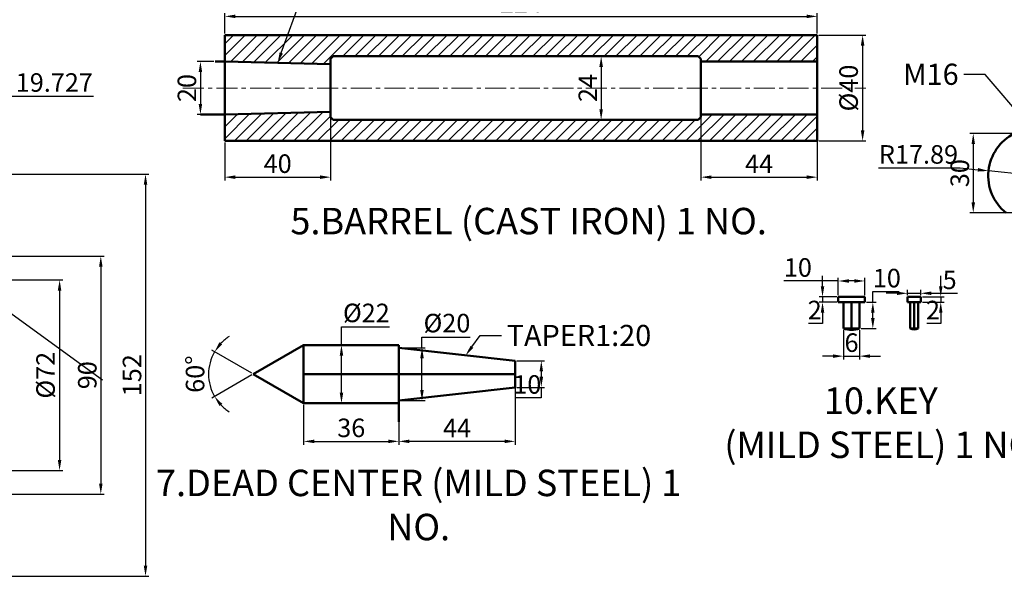
# Model space of a CAD drawing. Units: millimetres. Extents: x -66 to 1195, y -396 to 398.
# Tile 4 of 8: x 373 to 745, y -176 to 35. Entities that reach past the tile are written whole.
import ezdxf
from ezdxf import colors
from ezdxf.entities.mleader import LeaderData, LeaderLine
from ezdxf.math import Vec2, Vec3

# ---------------------------------------------------------------- set-up
doc = ezdxf.new("R2010")
doc.units = ezdxf.units.MM
doc.header["$LTSCALE"] = 0.5
doc.linetypes.add('CENTER', pattern=[50.8, 31.75, -6.35, 6.35, -6.35])
for name, color, linetype, lineweight in [('M-CNTR', 1, 'CENTER', 18), ('M-DIMS', 2, 'Continuous', 25), ('M-HATC', 8, 'Continuous', 18), ('M-OUTL', 7, 'Continuous', 50), ('M-TEXT', 7, 'Continuous', 25)]:
    doc.layers.add(name, color=color, linetype=linetype, lineweight=lineweight)
doc.styles.get("Standard").update_dxf_attribs({"font": 'arial.ttf'})
doc.dimstyles.new('ISO-25', dxfattribs={"dimtxt": 7, "dimasz": 4, "dimexe": 1.25, "dimexo": 0.625, "dimtad": 1, "dimtoh": 1, "dimtxsty": 'Standard', "dimcen": 2.5, "dimadec": 0, "dimazin": 0, "dimtfac": 1, "dimtmove": 0, "dimatfit": 3, "dimfxl": 1, "dimarcsym": 0})

# ---------------------------------------------------------------- blocks, each defined once
blk = doc.blocks.new('*D23')
at = {"layer": 'Defpoints', "color": 0, "ltscale": 0.5, "transparency": 16777216}
for p in [(346.94, -63.65), (346.94, -135.65), (387.75, -135.65)]:
    blk.add_point(p, dxfattribs=at)
at = {"layer": 'M-DIMS', "color": 0, "lineweight": -2, "ltscale": 0.5, "transparency": 16777216}
for p, q in [((347.56, -63.65), (389, -63.65)), ((387.75, -67.65), (387.75, -131.65)), ((347.56, -135.65), (389, -135.65))]:
    blk.add_line(p, q, dxfattribs=at)
at = {"layer": 'M-DIMS', "color": 0, "ltscale": 0.5, "transparency": 16777216}
for points in [[(387.08, -67.65), (388.41, -67.65), (387.75, -63.65)], [(387.08, -131.65), (388.41, -131.65), (387.75, -135.65)]]:
    blk.add_solid(points, dxfattribs=at)
at = {"layer": 'M-DIMS', "color": 0, "ltscale": 0.5, "transparency": 16777216, "insert": (383.35, -99.65), "char_height": 7, "attachment_point": 5, "rotation": 90}
blk.add_mtext('%%C72', dxfattribs=at)
blk = doc.blocks.new('*D24')
at = {"layer": 'Defpoints', "color": 0, "ltscale": 0.5, "transparency": 16777216}
for p in [(332.94, -54.65), (332.94, -144.65), (403.33, -144.65)]:
    blk.add_point(p, dxfattribs=at)
at = {"layer": 'M-DIMS', "color": 0, "lineweight": -2, "ltscale": 0.5, "transparency": 16777216}
for p, q in [((333.56, -54.65), (404.58, -54.65)), ((403.33, -58.65), (403.33, -140.65)), ((333.56, -144.65), (404.58, -144.65))]:
    blk.add_line(p, q, dxfattribs=at)
at = {"layer": 'M-DIMS', "color": 0, "ltscale": 0.5, "transparency": 16777216}
for points in [[(402.67, -58.65), (404, -58.65), (403.33, -54.65)], [(402.67, -140.65), (404, -140.65), (403.33, -144.65)]]:
    blk.add_solid(points, dxfattribs=at)
at = {"layer": 'M-DIMS', "color": 0, "ltscale": 0.5, "transparency": 16777216, "insert": (399.13, -99.65), "char_height": 7, "attachment_point": 5, "rotation": 90}
blk.add_mtext('90', dxfattribs=at)
blk = doc.blocks.new('*D25')
at = {"layer": 'Defpoints', "color": 0, "ltscale": 0.5, "transparency": 16777216}
for p in [(366.94, -23.65), (366.94, -175.65), (420.24, -175.65)]:
    blk.add_point(p, dxfattribs=at)
at = {"layer": 'M-DIMS', "color": 0, "lineweight": -2, "ltscale": 0.5, "transparency": 16777216}
for p, q in [((367.56, -23.65), (421.49, -23.65)), ((420.24, -27.65), (420.24, -171.65)), ((367.56, -175.65), (421.49, -175.65))]:
    blk.add_line(p, q, dxfattribs=at)
at = {"layer": 'M-DIMS', "color": 0, "ltscale": 0.5, "transparency": 16777216}
for points in [[(419.57, -27.65), (420.9, -27.65), (420.24, -23.65)], [(419.57, -171.65), (420.9, -171.65), (420.24, -175.65)]]:
    blk.add_solid(points, dxfattribs=at)
at = {"layer": 'M-DIMS', "color": 0, "ltscale": 0.5, "transparency": 16777216, "insert": (416.04, -99.65), "char_height": 7, "attachment_point": 5, "rotation": 90}
blk.add_mtext('152', dxfattribs=at)
blk = doc.blocks.new('*D47')
at = {"layer": 'Defpoints', "color": 0, "ltscale": 0.5, "transparency": 16777216}
for p in [(446.63, 18.9), (440.99, -1.1), (446.63, -1.1)]:
    blk.add_point(p, dxfattribs=at)
at = {"layer": 'M-DIMS', "color": 0, "lineweight": -2, "ltscale": 0.5, "transparency": 16777216}
for p, q in [((446, 18.9), (439.74, 18.9)), ((440.99, 14.9), (440.99, 2.9)), ((446, -1.1), (439.74, -1.1))]:
    blk.add_line(p, q, dxfattribs=at)
at = {"layer": 'M-DIMS', "color": 0, "ltscale": 0.5, "transparency": 16777216}
for points in [[(440.32, 14.9), (441.66, 14.9), (440.99, 18.9)], [(440.32, 2.9), (441.66, 2.9), (440.99, -1.1)]]:
    blk.add_solid(points, dxfattribs=at)
at = {"layer": 'M-DIMS', "color": 0, "ltscale": 0.5, "transparency": 16777216, "insert": (436.79, 8.9), "char_height": 7, "attachment_point": 5, "rotation": 90}
blk.add_mtext('20', dxfattribs=at)
blk = doc.blocks.new('*D48')
at = {"layer": 'Defpoints', "color": 0, "ltscale": 0.5, "transparency": 16777216}
for p in [(490.2, 8.9), (450.2, -11.1), (490.2, -24.79)]:
    blk.add_point(p, dxfattribs=at)
at = {"layer": 'M-DIMS', "color": 0, "lineweight": -2, "ltscale": 0.5, "transparency": 16777216}
for p, q in [((490.2, 8.28), (490.2, -26.04)), ((450.2, -11.72), (450.2, -26.04)), ((454.2, -24.79), (486.2, -24.79))]:
    blk.add_line(p, q, dxfattribs=at)
at = {"layer": 'M-DIMS', "color": 0, "ltscale": 0.5, "transparency": 16777216}
for points in [[(454.2, -24.12), (454.2, -25.46), (450.2, -24.79)], [(486.2, -24.12), (486.2, -25.46), (490.2, -24.79)]]:
    blk.add_solid(points, dxfattribs=at)
at = {"layer": 'M-DIMS', "color": 0, "ltscale": 0.5, "transparency": 16777216, "insert": (470.2, -20.59), "char_height": 7, "attachment_point": 5}
blk.add_mtext('40', dxfattribs=at)
blk = doc.blocks.new('*D49')
at = {"layer": 'Defpoints', "color": 0, "ltscale": 0.5, "transparency": 16777216}
for p in [(592.49, 20.9), (592.49, -3.1), (592.49, -3.1)]:
    blk.add_point(p, dxfattribs=at)
at = {"layer": 'M-DIMS', "color": 0, "lineweight": -2, "ltscale": 0.5, "transparency": 16777216}
for p, q in [((593.11, 20.9), (593.74, 20.9)), ((592.49, 16.9), (592.49, 0.9)), ((593.11, -3.1), (593.74, -3.1))]:
    blk.add_line(p, q, dxfattribs=at)
at = {"layer": 'M-DIMS', "color": 0, "ltscale": 0.5, "transparency": 16777216}
for points in [[(591.82, 16.9), (593.16, 16.9), (592.49, 20.9)], [(591.82, 0.9), (593.16, 0.9), (592.49, -3.1)]]:
    blk.add_solid(points, dxfattribs=at)
at = {"layer": 'M-DIMS', "color": 0, "ltscale": 0.5, "transparency": 16777216, "insert": (588.35, 8.9), "char_height": 7, "attachment_point": 5, "rotation": 90}
blk.add_mtext('24', dxfattribs=at)
blk = doc.blocks.new('*D50')
at = {"layer": 'Defpoints', "color": 0, "ltscale": 0.5, "transparency": 16777216}
for p in [(674.2, 35.99), (450.2, 28.9), (674.2, 28.9)]:
    blk.add_point(p, dxfattribs=at)
at = {"layer": 'M-DIMS', "color": 0, "lineweight": -2, "ltscale": 0.5, "transparency": 16777216}
for p, q in [((450.2, 29.53), (450.2, 37.24)), ((674.2, 29.53), (674.2, 37.24)), ((454.2, 35.99), (670.2, 35.99))]:
    blk.add_line(p, q, dxfattribs=at)
at = {"layer": 'M-DIMS', "color": 0, "ltscale": 0.5, "transparency": 16777216}
for points in [[(454.2, 36.65), (454.2, 35.32), (450.2, 35.99)], [(670.2, 36.65), (670.2, 35.32), (674.2, 35.99)]]:
    blk.add_solid(points, dxfattribs=at)
at = {"layer": 'M-DIMS', "color": 0, "ltscale": 0.5, "transparency": 16777216, "insert": (562.2, 40.13), "char_height": 7, "attachment_point": 5}
blk.add_mtext('224', dxfattribs=at)
blk = doc.blocks.new('*D51')
at = {"layer": 'Defpoints', "color": 0, "ltscale": 0.5, "transparency": 16777216}
for p in [(674.2, 28.9), (674.2, -11.1), (691.34, -11.1)]:
    blk.add_point(p, dxfattribs=at)
at = {"layer": 'M-DIMS', "color": 0, "lineweight": -2, "ltscale": 0.5, "transparency": 16777216}
for p, q in [((674.82, 28.9), (692.59, 28.9)), ((691.34, 24.9), (691.34, -7.1)), ((674.82, -11.1), (692.59, -11.1))]:
    blk.add_line(p, q, dxfattribs=at)
at = {"layer": 'M-DIMS', "color": 0, "ltscale": 0.5, "transparency": 16777216}
for points in [[(690.67, 24.9), (692.01, 24.9), (691.34, 28.9)], [(690.67, -7.1), (692.01, -7.1), (691.34, -11.1)]]:
    blk.add_solid(points, dxfattribs=at)
at = {"layer": 'M-DIMS', "color": 0, "ltscale": 0.5, "transparency": 16777216, "insert": (686.95, 8.9), "char_height": 7, "attachment_point": 5, "rotation": 90}
blk.add_mtext('%%C40', dxfattribs=at)
blk = doc.blocks.new('*D52')
at = {"layer": 'Defpoints', "color": 0, "ltscale": 0.5, "transparency": 16777216}
for p in [(630.2, 8.9), (674.2, 8.9), (674.2, -24.79)]:
    blk.add_point(p, dxfattribs=at)
at = {"layer": 'M-DIMS', "color": 0, "lineweight": -2, "ltscale": 0.5, "transparency": 16777216}
for p, q in [((630.2, 8.28), (630.2, -26.04)), ((674.2, 8.28), (674.2, -26.04)), ((634.2, -24.79), (670.2, -24.79))]:
    blk.add_line(p, q, dxfattribs=at)
at = {"layer": 'M-DIMS', "color": 0, "ltscale": 0.5, "transparency": 16777216}
for points in [[(634.2, -24.12), (634.2, -25.46), (630.2, -24.79)], [(670.2, -24.12), (670.2, -25.46), (674.2, -24.79)]]:
    blk.add_solid(points, dxfattribs=at)
at = {"layer": 'M-DIMS', "color": 0, "ltscale": 0.5, "transparency": 16777216, "insert": (652.2, -20.67), "char_height": 7, "attachment_point": 5}
blk.add_mtext('44', dxfattribs=at)
blk = doc.blocks.new('*D53')
at = {"layer": 'Defpoints', "color": 0, "ltscale": 0.5, "transparency": 16777216}
for p in [(516.01, -89.24), (516.01, -109.24), (524.75, -109.24)]:
    blk.add_point(p, dxfattribs=at)
at = {"layer": 'M-DIMS', "color": 0, "lineweight": -2, "ltscale": 0.5, "transparency": 16777216}
for p, q in [((524.75, -89.24), (524.75, -85.24)), ((524.75, -85.24), (543, -85.24)), ((516.64, -89.24), (526, -89.24)), ((524.75, -105.24), (524.75, -93.24)), ((516.64, -109.24), (526, -109.24))]:
    blk.add_line(p, q, dxfattribs=at)
at = {"layer": 'M-DIMS', "color": 0, "ltscale": 0.5, "transparency": 16777216}
for points in [[(524.09, -93.24), (525.42, -93.24), (524.75, -89.24)], [(524.09, -105.24), (525.42, -105.24), (524.75, -109.24)]]:
    blk.add_solid(points, dxfattribs=at)
at = {"layer": 'M-DIMS', "color": 0, "ltscale": 0.5, "transparency": 16777216, "insert": (534.19, -80.85), "char_height": 7, "attachment_point": 5}
blk.add_mtext('%%C20', dxfattribs=at)
blk = doc.blocks.new('*D54')
at = {"layer": 'Defpoints', "color": 0, "ltscale": 0.5, "transparency": 16777216}
for p in [(516.01, -99.24), (560.01, -99.24), (516.01, -124.65)]:
    blk.add_point(p, dxfattribs=at)
at = {"layer": 'M-DIMS', "color": 0, "lineweight": -2, "ltscale": 0.5, "transparency": 16777216}
for p, q in [((516.01, -99.87), (516.01, -125.9)), ((560.01, -99.87), (560.01, -125.9)), ((556.01, -124.65), (520.01, -124.65))]:
    blk.add_line(p, q, dxfattribs=at)
at = {"layer": 'M-DIMS', "color": 0, "ltscale": 0.5, "transparency": 16777216}
for points in [[(520.01, -123.99), (520.01, -125.32), (516.01, -124.65)], [(556.01, -123.99), (556.01, -125.32), (560.01, -124.65)]]:
    blk.add_solid(points, dxfattribs=at)
at = {"layer": 'M-DIMS', "color": 0, "ltscale": 0.5, "transparency": 16777216, "insert": (538.01, -120.53), "char_height": 7, "attachment_point": 5}
blk.add_mtext('44', dxfattribs=at)
blk = doc.blocks.new('*D55')
at = {"layer": 'Defpoints', "color": 0, "ltscale": 0.5, "transparency": 16777216}
for p in [(480.01, -88.24), (480.01, -110.24), (494.31, -110.24)]:
    blk.add_point(p, dxfattribs=at)
at = {"layer": 'M-DIMS', "color": 0, "lineweight": -2, "ltscale": 0.5, "transparency": 16777216}
for p, q in [((494.31, -88.24), (494.31, -81.4)), ((494.31, -81.4), (512.51, -81.4)), ((480.64, -88.24), (495.56, -88.24)), ((494.31, -106.24), (494.31, -92.24)), ((480.64, -110.24), (495.56, -110.24))]:
    blk.add_line(p, q, dxfattribs=at)
at = {"layer": 'M-DIMS', "color": 0, "ltscale": 0.5, "transparency": 16777216}
for points in [[(493.65, -92.24), (494.98, -92.24), (494.31, -88.24)], [(493.65, -106.24), (494.98, -106.24), (494.31, -110.24)]]:
    blk.add_solid(points, dxfattribs=at)
at = {"layer": 'M-DIMS', "color": 0, "ltscale": 0.5, "transparency": 16777216, "insert": (503.72, -77.01), "char_height": 7, "attachment_point": 5}
blk.add_mtext('%%C22', dxfattribs=at)
blk = doc.blocks.new('*D56')
at = {"layer": 'Defpoints', "color": 0, "ltscale": 0.5, "transparency": 16777216}
for p in [(480.01, -110.24), (516.01, -110.24), (516.01, -124.65)]:
    blk.add_point(p, dxfattribs=at)
at = {"layer": 'M-DIMS', "color": 0, "lineweight": -2, "ltscale": 0.5, "transparency": 16777216}
for p, q in [((480.01, -110.87), (480.01, -125.9)), ((516.01, -110.87), (516.01, -125.9)), ((484.01, -124.65), (512.01, -124.65))]:
    blk.add_line(p, q, dxfattribs=at)
at = {"layer": 'M-DIMS', "color": 0, "ltscale": 0.5, "transparency": 16777216}
for points in [[(484.01, -123.99), (484.01, -125.32), (480.01, -124.65)], [(512.01, -123.99), (512.01, -125.32), (516.01, -124.65)]]:
    blk.add_solid(points, dxfattribs=at)
at = {"layer": 'M-DIMS', "color": 0, "ltscale": 0.5, "transparency": 16777216, "insert": (498.01, -120.45), "char_height": 7, "attachment_point": 5}
blk.add_mtext('36', dxfattribs=at)
blk = doc.blocks.new('*D57')
at = {"layer": 'Defpoints', "color": 0, "ltscale": 0.5, "transparency": 16777216}
for p in [(480.01, -88.24), (444.32, -96.31), (460.96, -99.24), (460.96, -99.24), (480.01, -110.24)]:
    blk.add_point(p, dxfattribs=at)
at = {"layer": 'M-DIMS', "color": 0, "lineweight": -2, "ltscale": 0.5, "transparency": 16777216}
for p, q in [((460.42, -98.93), (445.25, -90.17)), ((460.42, -99.56), (445.25, -108.32))]:
    blk.add_line(p, q, dxfattribs=at)
for start, end in [(122.8038, 136.4019), (150, 210), (223.5981, 237.1962)]:
    blk.add_arc((460.96, -99.24), 16.89, start, end, dxfattribs=at)
at = {"layer": 'M-DIMS', "color": 0, "ltscale": 0.5, "transparency": 16777216}
for points in [[(449.26, -87.99), (448.19, -87.19), (446.33, -90.8)], [(448.19, -111.29), (449.26, -110.49), (446.33, -107.69)]]:
    blk.add_solid(points, dxfattribs=at)
at = {"layer": 'M-DIMS', "color": 0, "ltscale": 0.5, "transparency": 16777216, "insert": (439.87, -99.24), "char_height": 7, "attachment_point": 5, "rotation": 90}
blk.add_mtext('60°', dxfattribs=at)
blk = doc.blocks.new('*D58')
at = {"layer": 'Defpoints', "color": 0, "ltscale": 0.5, "transparency": 16777216}
for p in [(682.15, -70.05), (676.19, -72.05), (682.15, -72.05)]:
    blk.add_point(p, dxfattribs=at)
at = {"layer": 'M-DIMS', "color": 0, "lineweight": -2, "ltscale": 0.5, "transparency": 16777216}
for p, q in [((676.19, -66.05), (676.19, -62.05)), ((681.53, -70.05), (674.94, -70.05)), ((676.19, -70.05), (676.19, -72.05)), ((681.53, -72.05), (674.94, -72.05)), ((676.19, -76.05), (676.19, -80.05)), ((676.19, -80.05), (670.93, -80.05))]:
    blk.add_line(p, q, dxfattribs=at)
at = {"layer": 'M-DIMS', "color": 0, "ltscale": 0.5, "transparency": 16777216}
for points in [[(675.52, -66.05), (676.85, -66.05), (676.19, -70.05)], [(675.52, -76.05), (676.85, -76.05), (676.19, -72.05)]]:
    blk.add_solid(points, dxfattribs=at)
at = {"layer": 'M-DIMS', "color": 0, "ltscale": 0.5, "transparency": 16777216, "insert": (673.24, -75.91), "char_height": 7, "attachment_point": 5}
blk.add_mtext('2', dxfattribs=at)
blk = doc.blocks.new('*D59')
at = {"layer": 'Defpoints', "color": 0, "ltscale": 0.5, "transparency": 16777216}
for p in [(692.15, -64.03), (682.15, -70.05), (692.15, -70.05)]:
    blk.add_point(p, dxfattribs=at)
at = {"layer": 'M-DIMS', "color": 0, "lineweight": -2, "ltscale": 0.5, "transparency": 16777216}
for p, q in [((682.15, -69.43), (682.15, -62.78)), ((692.15, -69.43), (692.15, -62.78)), ((682.15, -64.03), (661.56, -64.03)), ((688.15, -64.03), (686.15, -64.03))]:
    blk.add_line(p, q, dxfattribs=at)
at = {"layer": 'M-DIMS', "color": 0, "ltscale": 0.5, "transparency": 16777216}
for points in [[(686.15, -63.36), (686.15, -64.7), (682.15, -64.03)], [(688.15, -63.36), (688.15, -64.7), (692.15, -64.03)]]:
    blk.add_solid(points, dxfattribs=at)
at = {"layer": 'M-DIMS', "color": 0, "ltscale": 0.5, "transparency": 16777216, "insert": (666.86, -59.83), "char_height": 7, "attachment_point": 5}
blk.add_mtext('10', dxfattribs=at)
blk = doc.blocks.new('*D60')
at = {"layer": 'Defpoints', "color": 0, "ltscale": 0.5, "transparency": 16777216}
for p in [(684.15, -82.05), (690.15, -82.05), (690.15, -92.44)]:
    blk.add_point(p, dxfattribs=at)
at = {"layer": 'M-DIMS', "color": 0, "lineweight": -2, "ltscale": 0.5, "transparency": 16777216}
for p, q in [((684.15, -82.68), (684.15, -93.69)), ((690.15, -82.68), (690.15, -93.69)), ((680.15, -92.44), (676.15, -92.44)), ((684.15, -92.44), (690.15, -92.44)), ((694.15, -92.44), (698.15, -92.44))]:
    blk.add_line(p, q, dxfattribs=at)
at = {"layer": 'M-DIMS', "color": 0, "ltscale": 0.5, "transparency": 16777216}
for points in [[(680.15, -91.77), (680.15, -93.1), (684.15, -92.44)], [(694.15, -91.77), (694.15, -93.1), (690.15, -92.44)]]:
    blk.add_solid(points, dxfattribs=at)
at = {"layer": 'M-DIMS', "color": 0, "ltscale": 0.5, "transparency": 16777216, "insert": (687.15, -88.24), "char_height": 7, "attachment_point": 5}
blk.add_mtext('6', dxfattribs=at)
blk = doc.blocks.new('*D61')
at = {"layer": 'Defpoints', "color": 0, "ltscale": 0.5, "transparency": 16777216}
for p in [(692.15, -72.05), (695.2, -72.05), (690.15, -82.05)]:
    blk.add_point(p, dxfattribs=at)
at = {"layer": 'M-DIMS', "color": 0, "lineweight": -2, "ltscale": 0.5, "transparency": 16777216}
for p, q in [((695.2, -72.05), (695.2, -68.05)), ((695.2, -68.05), (705.17, -68.05)), ((692.78, -72.05), (696.45, -72.05)), ((695.2, -78.05), (695.2, -76.05)), ((690.78, -82.05), (696.45, -82.05))]:
    blk.add_line(p, q, dxfattribs=at)
at = {"layer": 'M-DIMS', "color": 0, "ltscale": 0.5, "transparency": 16777216}
for points in [[(694.53, -76.05), (695.86, -76.05), (695.2, -72.05)], [(694.53, -78.05), (695.86, -78.05), (695.2, -82.05)]]:
    blk.add_solid(points, dxfattribs=at)
at = {"layer": 'M-DIMS', "color": 0, "ltscale": 0.5, "transparency": 16777216, "insert": (700.49, -63.85), "char_height": 7, "attachment_point": 5}
blk.add_mtext('10', dxfattribs=at)
blk = doc.blocks.new('*D62')
at = {"layer": 'Defpoints', "color": 0, "ltscale": 0.5, "transparency": 16777216}
for p in [(713.29, -70.05), (713.29, -72.05), (720.88, -72.05)]:
    blk.add_point(p, dxfattribs=at)
at = {"layer": 'M-DIMS', "color": 0, "lineweight": -2, "ltscale": 0.5, "transparency": 16777216}
for p, q in [((720.88, -66.05), (720.88, -62.05)), ((713.92, -70.05), (722.13, -70.05)), ((720.88, -70.05), (720.88, -72.05)), ((713.92, -72.05), (722.13, -72.05)), ((720.88, -76.05), (720.88, -80.05)), ((720.88, -80.05), (715.62, -80.05))]:
    blk.add_line(p, q, dxfattribs=at)
at = {"layer": 'M-DIMS', "color": 0, "ltscale": 0.5, "transparency": 16777216}
for points in [[(720.22, -66.05), (721.55, -66.05), (720.88, -70.05)], [(720.22, -76.05), (721.55, -76.05), (720.88, -72.05)]]:
    blk.add_solid(points, dxfattribs=at)
at = {"layer": 'M-DIMS', "color": 0, "ltscale": 0.5, "transparency": 16777216, "insert": (717.94, -75.91), "char_height": 7, "attachment_point": 5}
blk.add_mtext('2', dxfattribs=at)
blk = doc.blocks.new('*D63')
at = {"layer": 'Defpoints', "color": 0, "ltscale": 0.5, "transparency": 16777216}
for p in [(708.29, -70.05), (713.29, -68.68), (713.29, -70.05)]:
    blk.add_point(p, dxfattribs=at)
at = {"layer": 'M-DIMS', "color": 0, "lineweight": -2, "ltscale": 0.5, "transparency": 16777216}
for p, q in [((704.29, -68.68), (700.29, -68.68)), ((708.29, -69.43), (708.29, -67.43)), ((708.29, -68.68), (713.29, -68.68)), ((713.29, -69.43), (713.29, -67.43)), ((717.29, -68.68), (727.18, -68.68))]:
    blk.add_line(p, q, dxfattribs=at)
at = {"layer": 'M-DIMS', "color": 0, "ltscale": 0.5, "transparency": 16777216}
for points in [[(704.29, -68.01), (704.29, -69.35), (708.29, -68.68)], [(717.29, -68.01), (717.29, -69.35), (713.29, -68.68)]]:
    blk.add_solid(points, dxfattribs=at)
at = {"layer": 'M-DIMS', "color": 0, "ltscale": 0.5, "transparency": 16777216, "insert": (724.24, -64.5), "char_height": 7, "attachment_point": 5}
blk.add_mtext('5', dxfattribs=at)
blk = doc.blocks.new('*D75')
at = {"layer": 'Defpoints', "color": 0, "ltscale": 0.5, "transparency": 16777216}
for p in [(756.72, -8.28), (733.17, -38.28), (755.15, -38.28)]:
    blk.add_point(p, dxfattribs=at)
at = {"layer": 'M-DIMS', "color": 0, "lineweight": -2, "ltscale": 0.5, "transparency": 16777216}
for p, q in [((756.1, -8.28), (731.92, -8.28)), ((733.17, -12.28), (733.17, -34.28)), ((754.53, -38.28), (731.92, -38.28))]:
    blk.add_line(p, q, dxfattribs=at)
at = {"layer": 'M-DIMS', "color": 0, "ltscale": 0.5, "transparency": 16777216}
for points in [[(732.51, -12.28), (733.84, -12.28), (733.17, -8.28)], [(732.51, -34.28), (733.84, -34.28), (733.17, -38.28)]]:
    blk.add_solid(points, dxfattribs=at)
at = {"layer": 'M-DIMS', "color": 0, "ltscale": 0.5, "transparency": 16777216, "insert": (728.97, -23.28), "char_height": 7, "attachment_point": 5, "rotation": 90}
blk.add_mtext('30', dxfattribs=at)
blk = doc.blocks.new('*D106')
at = {"layer": 'Defpoints', "color": 0, "ltscale": 0.5, "transparency": 16777216}
for p in [(366.94, 5.88), (347.21, -23.65), (366.94, -23.65)]:
    blk.add_point(p, dxfattribs=at)
at = {"layer": 'M-DIMS', "color": 0, "lineweight": -2, "ltscale": 0.5, "transparency": 16777216}
for p, q in [((347.21, -23.03), (347.21, 7.13)), ((351.21, 5.88), (362.94, 5.88)), ((366.94, -23.03), (366.94, 7.13)), ((366.94, 5.88), (400.59, 5.88))]:
    blk.add_line(p, q, dxfattribs=at)
at = {"layer": 'M-DIMS', "color": 0, "ltscale": 0.5, "transparency": 16777216}
for points in [[(351.21, 6.55), (351.21, 5.21), (347.21, 5.88)], [(362.94, 6.55), (362.94, 5.21), (366.94, 5.88)]]:
    blk.add_solid(points, dxfattribs=at)
at = {"layer": 'M-DIMS', "color": 0, "ltscale": 0.5, "transparency": 16777216, "insert": (385.76, 10.08), "char_height": 7, "attachment_point": 5}
blk.add_mtext('19.727', dxfattribs=at)
blk = doc.blocks.new('*D107')
at = {"layer": 'Defpoints', "color": 0, "ltscale": 0.5, "transparency": 16777216}
for p in [(560.01, -94.24), (560.01, -104.24), (569.86, -104.24)]:
    blk.add_point(p, dxfattribs=at)
at = {"layer": 'M-DIMS', "color": 0, "lineweight": -2, "ltscale": 0.5, "transparency": 16777216}
for p, q in [((560.64, -94.24), (571.11, -94.24)), ((569.86, -98.24), (569.86, -100.24)), ((560.64, -104.24), (571.11, -104.24)), ((569.86, -104.24), (569.86, -108.24)), ((569.86, -108.24), (559.89, -108.24))]:
    blk.add_line(p, q, dxfattribs=at)
at = {"layer": 'M-DIMS', "color": 0, "ltscale": 0.5, "transparency": 16777216}
for points in [[(569.2, -98.24), (570.53, -98.24), (569.86, -94.24)], [(569.2, -100.24), (570.53, -100.24), (569.86, -104.24)]]:
    blk.add_solid(points, dxfattribs=at)
at = {"layer": 'M-DIMS', "color": 0, "ltscale": 0.5, "transparency": 16777216, "insert": (564.57, -104.04), "char_height": 7, "attachment_point": 5}
blk.add_mtext('10', dxfattribs=at)
blk = doc.blocks.new('*D121')
at = {"layer": 'Defpoints', "color": 0, "ltscale": 0.5, "transparency": 16777216}
for p in [(325.99, -44.9), (403.98, -101.56)]:
    blk.add_point(p, dxfattribs=at)
at = {"layer": 'M-DIMS', "color": 0, "lineweight": -2, "ltscale": 0.5, "transparency": 16777216}
for p, q in [((253.72, -10.91), (279.2, -10.91)), ((279.2, -10.91), (322.76, -42.55)), ((403.98, -101.56), (325.99, -44.9))]:
    blk.add_line(p, q, dxfattribs=at)
at = {"layer": 'M-DIMS', "color": 0, "ltscale": 0.5, "transparency": 16777216}
blk.add_solid([(323.15, -42.01), (322.36, -43.09), (325.99, -44.9)], dxfattribs=at)
at = {"layer": 'M-DIMS', "color": 0, "ltscale": 0.5, "transparency": 16777216, "insert": (266.15, -6.71), "char_height": 7, "attachment_point": 5}
blk.add_mtext('R96.4', dxfattribs=at)
blk = doc.blocks.new('*D132')
at = {"layer": 'Defpoints', "color": 0, "ltscale": 0.5, "transparency": 16777216}
for p in [(738.93, -22.42), (756.72, -24.28)]:
    blk.add_point(p, dxfattribs=at)
at = {"layer": 'M-DIMS', "color": 0, "lineweight": -2, "ltscale": 0.5, "transparency": 16777216}
for p, q in [((697.29, -21.3), (728.25, -21.3)), ((728.25, -21.3), (734.95, -22)), ((756.72, -24.28), (738.93, -22.42))]:
    blk.add_line(p, q, dxfattribs=at)
at = {"layer": 'M-DIMS', "color": 0, "ltscale": 0.5, "transparency": 16777216}
blk.add_solid([(735.02, -21.34), (734.88, -22.67), (738.93, -22.42)], dxfattribs=at)
at = {"layer": 'M-DIMS', "color": 0, "ltscale": 0.5, "transparency": 16777216, "insert": (712.46, -17.1), "char_height": 7, "attachment_point": 5}
blk.add_mtext('R17.89', dxfattribs=at)

msp = doc.modelspace()

# ---------------------------------------------------------------- hatches: boundary and pattern name
at = {"layer": 'M-HATC', "ltscale": 0.5}
h = msp.add_hatch(dxfattribs=at)
h.set_pattern_fill('ANSI31', color=256)
h.set_pattern_definition([(45, (-203.5867, 63.3575), (-2.245064, 2.245064), [])])
h.paths.add_polyline_path([(490.1953, 17.9037), (490.1953, 18.9037), (490.1953, 19.9037), (491.1953, 20.9037), (629.1953, 20.9037), (630.1953, 19.9037), (630.1953, 18.9037), (674.1953, 18.9037), (674.1953, 28.9037), (450.1953, 28.9037), (450.1953, 18.9037)])
h.paths.add_polyline_path([(450.1953, -1.0963), (450.1953, -11.0963), (674.1953, -11.0963), (674.1953, -1.0963), (630.1953, -1.0963), (630.1953, -2.0963), (629.1953, -3.0963), (491.1953, -3.0963), (490.1953, -2.0963), (490.1953, -0.0963)])

# ---------------------------------------------------------------- linework, layer by layer
at = {"layer": 'M-CNTR', "ltscale": 0.5}
msp.add_line((434.3388, 8.9037), (692.5309, 8.9037), dxfattribs=at)
at = {"layer": 'M-OUTL', "ltscale": 0.5}
for p, q in [((450.1953, 28.9037), (450.1953, -11.0963)), ((674.1953, 28.9037), (450.1953, 28.9037)), ((674.1953, -11.0963), (674.1953, 28.9037)), ((450.1953, 18.9037), (446.6283, 18.9037)), ((450.1953, 18.9037), (490.1953, 17.9037)), ((491.1953, 20.9037), (490.1953, 19.9037)), ((490.1953, 8.9037), (490.1953, 19.9037)), ((490.1953, 18.9037), (490.1953, 17.9037)), ((491.1953, 20.9037), (629.1953, 20.9037)), ((629.1953, 20.9037), (630.1953, 19.9037)), ((630.1953, -2.0963), (630.1953, 19.9037)), ((630.1953, 18.9037), (674.1953, 18.9037)), ((490.1953, 8.9037), (490.1953, -2.0963)), ((450.1953, -1.0963), (440.9896, -1.0963)), ((450.1953, -1.0963), (490.1953, -0.0963)), ((490.1953, -2.0963), (491.1953, -3.0963)), ((491.1953, -3.0963), (629.1953, -3.0963)), ((630.1953, -2.0963), (629.1953, -3.0963)), ((630.1953, -1.0963), (674.1953, -1.0963)), ((450.1953, -11.0963), (674.1953, -11.0963)), ((682.1529, -70.0503), (692.1529, -70.0503)), ((682.1529, -72.0503), (682.1529, -70.0503)), ((692.1529, -70.0503), (692.1529, -72.0503)), ((708.2926, -70.0503), (713.2926, -70.0503)), ((708.2926, -72.0503), (708.2926, -70.0503)), ((713.2926, -70.0503), (713.2926, -72.0503)), ((692.1529, -72.0503), (682.1529, -72.0503)), ((684.1529, -82.0503), (684.1529, -72.0503)), ((687.1529, -72.0503), (687.1529, -82.0503)), ((690.1529, -82.0503), (690.1529, -72.0503)), ((713.2926, -72.0503), (708.2926, -72.0503)), ((709.2926, -82.0503), (709.2926, -72.0503)), ((710.7926, -72.0503), (710.7926, -82.0503)), ((712.2926, -82.0503), (712.2926, -72.0503)), ((687.1529, -82.0503), (684.1529, -82.0503)), ((687.1529, -82.0503), (690.1529, -82.0503)), ((710.7926, -82.0503), (709.2926, -82.0503)), ((710.7926, -82.0503), (712.2926, -82.0503)), ((480.0135, -88.2433), (460.961, -99.2433)), ((480.0135, -88.2433), (480.0135, -110.2433)), ((516.0135, -88.2433), (480.0135, -88.2433)), ((516.0135, -117.2433), (516.0135, -88.2433)), ((516.0135, -89.2433), (560.0135, -94.2433)), ((560.0135, -104.2433), (560.0135, -94.2433)), ((480.0135, -110.2433), (460.961, -99.2433)), ((516.0135, -99.2433), (480.0135, -99.2433)), ((516.0135, -99.2433), (560.0135, -99.2433)), ((516.0135, -109.2433), (560.0135, -104.2433)), ((516.0135, -110.2433), (480.0135, -110.2433))]:
    msp.add_line(p, q, dxfattribs=at)
for centre, radius, start, end in [((756.72, -24.2825), 17.8885, 116.565051, 231.501439), ((687.1529, -71.9068), 10.5779, 253.524218, 286.475782), ((710.7926, -77.7524), 4.5522, 250.76096, 289.23904)]:
    msp.add_arc(centre, radius, start, end, dxfattribs=at)

# ---------------------------------------------------------------- texts
at = {"layer": 'M-TEXT', "ltscale": 0.5, "char_height": 10, "attachment_point": 1}
for s, insert in [('\\pxqc;5.BARREL (CAST IRON) 1 NO.', (463.0851, -36.3836)), ('\\pxqc;10.KEY\\P (MILD STEEL) 1 NO.', (596.2267, -104.2757)), ('\\pxqc;7.DEAD CENTER (MILD STEEL) 1 NO.', (421.5098, -135.3578))]:
    msp.add_mtext_dynamic_manual_height_columns(s, width=203.992441, gutter_width=12.5, heights=[0], dxfattribs=dict(at, insert=insert))

# ---------------------------------------------------------------- dimensions: what is measured, and where the dimension line sits
at = {"layer": 'M-DIMS', "ltscale": 0.5}
for base, p1, p2, override, picture, middle in [((674.1953, 35.9864), (450.1953, 28.9037), (674.1953, 28.9037), {"dimclrd": 0, "dimclre": 0, "dimclrt": 0}, '*D50', (562.1953, 40.1258)), ((366.9367, 5.8791), (347.2095, -23.6533), (366.9367, -23.6533), {"dimdec": 3, "dimlfac": 1, "dimrnd": 0, "dimzin": 0, "dimdsep": 46, "dimlunit": 2}, '*D106', (385.7622, 10.0781)), ((490.1953, -24.7902), (450.1953, -11.0963), (490.1953, 8.9037), {"dimclrd": 0, "dimclre": 0, "dimclrt": 0}, '*D48', (470.1953, -20.5912)), ((674.1953, -24.7902), (630.1953, 8.9037), (674.1953, 8.9037), {"dimclrd": 0, "dimclre": 0, "dimclrt": 0}, '*D52', (652.1953, -20.6652)), ((713.2926, -68.6802), (708.2926, -70.0503), (713.2926, -70.0503), {"dimclrd": 0, "dimclre": 0, "dimclrt": 0}, '*D63', (724.2382, -64.4955)), ((690.1529, -92.4357), (684.1529, -82.0503), (690.1529, -82.0503), {"dimclrd": 0, "dimclre": 0, "dimclrt": 0}, '*D60', (687.1529, -88.2367)), ((516.0135, -124.6519), (560.0135, -99.2433), (516.0135, -99.2433), {"dimclrd": 0, "dimclre": 0, "dimclrt": 0}, '*D54', (538.0135, -120.5269)), ((516.0135, -124.6519), (480.0135, -110.2433), (516.0135, -110.2433), {"dimclrd": 0, "dimclre": 0, "dimclrt": 0}, '*D56', (498.0135, -120.4505))]:
    dim = msp.add_linear_dim(base=base, p1=p1, p2=p2, dimstyle='ISO-25', override=override, dxfattribs=at)
    dim.commit()
    dim.dimension.update_dxf_attribs({"geometry": picture, "text_midpoint": middle})
for base, p1, p2, picture, middle in [((691.3405, -11.0963), (674.1953, 28.9037), (674.1953, -11.0963), '*D51', (686.9457, 8.9037)), ((387.7471, -135.6533), (346.9367, -63.6533), (346.9367, -135.6533), '*D23', (383.3523, -99.6533))]:
    dim = msp.add_linear_dim(base=base, p1=p1, p2=p2, angle=90, text='%%C<>', dimstyle='ISO-25', override={"dimclrd": 0, "dimclre": 0, "dimclrt": 0}, dxfattribs=at)
    dim.commit()
    dim.dimension.update_dxf_attribs({"geometry": picture, "text_midpoint": middle})
for base, p1, p2, override, picture, middle in [((440.9896, -1.0963), (446.6283, 18.9037), (446.6283, -1.0963), {"dimclrd": 0, "dimclre": 0, "dimclrt": 0}, '*D47', (436.7906, 8.9037)), ((592.4887, -3.0963), (592.4887, 20.9037), (592.4887, -3.0963), {"dimclrd": 0, "dimclre": 0, "dimclrt": 0}, '*D49', (588.3494, 8.9037)), ((733.173, -38.2825), (756.72, -8.2825), (755.1523, -38.2825), {"dimclrd": 0, "dimclre": 0, "dimclrt": 0}, '*D75', (728.9716, -23.2825)), ((420.2377, -175.6533), (366.9367, -23.6533), (366.9367, -175.6533), {"dimclrd": 0, "dimclre": 0, "dimclrt": 0}, '*D25', (416.0387, -99.6533)), ((403.3318, -144.6533), (332.9367, -54.6533), (332.9367, -144.6533), {"dimclrd": 0, "dimclre": 0, "dimclrt": 0}, '*D24', (399.1328, -99.6533)), ((695.1969, -72.0503), (690.1529, -82.0503), (692.1529, -72.0503), {"dimclrd": 0, "dimclre": 0, "dimclrt": 0}, '*D61', (700.4942, -63.8513)), ((676.1874, -72.0503), (682.1529, -70.0503), (682.1529, -72.0503), {"dimclrd": 0, "dimclre": 0, "dimclrt": 0}, '*D58', (673.2442, -75.911)), ((720.882, -72.0503), (713.2926, -70.0503), (713.2926, -72.0503), {"dimclrd": 0, "dimclre": 0, "dimclrt": 0}, '*D62', (717.9388, -75.911)), ((569.8635, -104.2433), (560.0135, -94.2433), (560.0135, -104.2433), {"dimdec": 0, "dimlfac": 1, "dimrnd": 0, "dimzin": 0, "dimdsep": 46, "dimlunit": 2}, '*D107', (564.5663, -104.0443))]:
    dim = msp.add_linear_dim(base=base, p1=p1, p2=p2, angle=90, dimstyle='ISO-25', override=override, dxfattribs=at)
    dim.commit()
    dim.dimension.update_dxf_attribs({"geometry": picture, "text_midpoint": middle})
for center, mpoint, override, picture, middle in [((403.9811, -101.5567), (325.9927, -44.9019), {"dimdec": 1, "dimlfac": 1, "dimrnd": 0, "dimzin": 0, "dimdsep": 46, "dimlunit": 2}, '*D121', (266.1479, -10.909)), ((756.72, -24.2825), (738.9287, -22.4199), {"dimdec": 2, "dimlfac": 1, "dimrnd": 0, "dimzin": 0, "dimdsep": 46, "dimlunit": 2}, '*D132', (728.2539, -21.3023))]:
    dim = msp.add_radius_dim(center=center, mpoint=mpoint, dimstyle='ISO-25', override=override, dxfattribs=at)
    dim.commit()
    dim.dimension.update_dxf_attribs({"geometry": picture, "text_midpoint": middle, "dimtype": 164})
dim = msp.add_linear_dim(base=(692.1529, -64.0293), p1=(682.1529, -70.0503), p2=(692.1529, -70.0503), dimstyle='ISO-25', override={"dimclrd": 0, "dimclre": 0, "dimclrt": 0}, dxfattribs=at)
dim.commit()
dim.dimension.update_dxf_attribs({"geometry": '*D59', "text_midpoint": (666.8594, -64.0293), "dimtype": 160})
for base, p1, p2, picture, middle in [((494.3142, -110.2433), (480.0135, -88.2433), (480.0135, -110.2433), '*D55', (503.725, -81.4042)), ((524.7546, -109.2433), (516.0135, -89.2433), (516.0135, -109.2433), '*D53', (534.1893, -85.2433))]:
    dim = msp.add_linear_dim(base=base, p1=p1, p2=p2, angle=90, text='%%C<>', dimstyle='ISO-25', override={"dimclrd": 0, "dimclre": 0, "dimclrt": 0}, dxfattribs=at)
    dim.commit()
    dim.dimension.update_dxf_attribs({"geometry": picture, "text_midpoint": middle, "dimtype": 160})
dim = msp.add_angular_dim_2l(base=(444.324, -96.3097), line1=((480.0135, -110.2433), (460.961, -99.2433)), line2=((480.0135, -88.2433), (460.961, -99.2433)), dimstyle='ISO-25', override={"dimclrd": 0, "dimclre": 0, "dimclrt": 0}, dxfattribs=at)
dim.commit()
dim.dimension.update_dxf_attribs({"geometry": '*D57', "text_midpoint": (439.8683, -99.2433)})

# ---------------------------------------------------------------- leaders
at = {"layer": 'M-TEXT', "ltscale": 0.5}
ml = msp.add_multileader_mtext('Standard', dxfattribs=at)
ml.set_content('TAPER1:20', color=256)
ml.set_leader_properties()
ml.build(insert=Vec2(0, 0))
ctx = ml.context
ctx.base_point, ctx.char_height, ctx.plane_origin = Vec3(489.22, 48.8808), 8, Vec3(470.1953, 18.4037)
notes = []
notes.append((ctx, [(0, (1, 1, 0), (481.22, 48.8808), (1, 0), 8, [(0, [(470.1953, 18.4037)], 0, [])])]))
ctx.mtext.insert, ctx.mtext.flow_direction = Vec3(491.22, 52.949), 5
ml = msp.add_multileader_mtext('Standard', dxfattribs=at)
ml.set_content('M16', color=256)
ml.set_leader_properties()
ml.build(insert=Vec2(0, 0))
ctx = ml.context
ctx.base_point, ctx.char_height, ctx.plane_origin = Vec3(705.2463, 14.0391), 8, Vec3(756.72, -8.2825)
ctx.text_align_type = 2
notes.append((ctx, [(0, (1, 1, 0), (737.6447, 14.0391), (-1, 0), 8, [(0, [(756.72, -8.2825)], 0, [])])]))
ctx.mtext.insert, ctx.mtext.alignment, ctx.mtext.flow_direction = Vec3(727.6447, 18.1073), 3, 5
ml = msp.add_multileader_mtext('Standard', dxfattribs=at)
ml.set_content('TAPER1:20', color=256)
ml.set_leader_properties()
ml.build(insert=Vec2(0, 0))
ctx = ml.context
ctx.base_point, ctx.char_height, ctx.plane_origin = Vec3(554.7869, -84.6898), 8, Vec3(541.2722, -92.1136)
notes.append((ctx, [(0, (1, 1, 0), (546.7869, -84.6898), (1, 0), 8, [(0, [(541.2722, -92.1136)], 0, [])])]))
ctx.mtext.insert, ctx.mtext.flow_direction = Vec3(556.7869, -80.6216), 5
for ctx, leaders in notes:
    for number, flags, end, landing, length, lines in leaders:
        leader = LeaderData()
        leader.index, (leader.has_last_leader_line, leader.has_dogleg_vector, leader.attachment_direction) = number, flags
        leader.last_leader_point, leader.dogleg_vector, leader.dogleg_length = Vec3(end), Vec3(landing), length
        for number, points, colour, breaks in lines:
            line = LeaderLine()
            line.index, line.vertices, line.color, line.breaks = number, Vec3.list(points), colors.encode_raw_color(colour), breaks
            leader.lines.append(line)
        ctx.leaders.append(leader)

doc.saveas('drawing.dxf')
